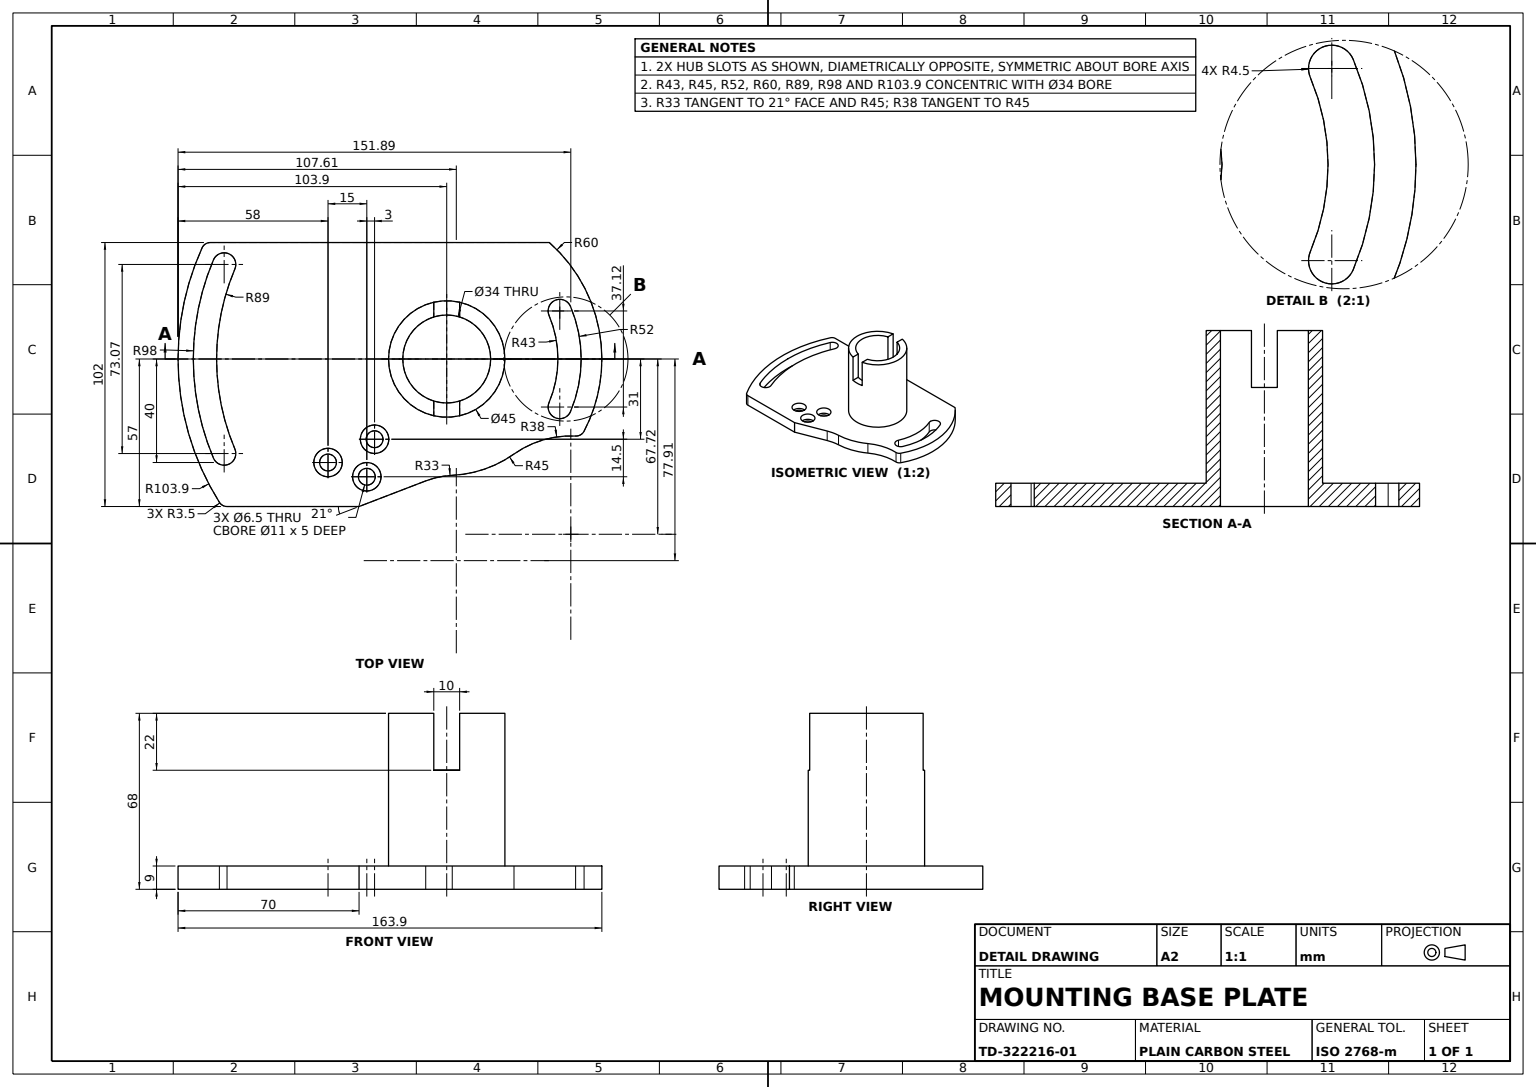
SolidWorks part; units mm, degrees
material "Plain Carbon Steel"
ref_plane "Front Plane" through (0, 0, 0) normal (0, 0, 1) x (1, 0, 0)
ref_plane "Top Plane" through (0, 0, 0) normal (0, 1, 0) x (1, 0, 0)
ref_plane "Right Plane" through (0, 0, 0) normal (1, 0, 0) x (0, 0, -1)
sketch "Cam Plate Profile" plane through (0, 0, 0) normal (0, 1, 0) x (1, 0, 0)
  line L0 (0, 0) -> (-45, 0) construction
  line L1 (-45, 39.6857) -> (-45, -91.4216)
  line L2 (0, 96.201) -> (0, -121.4761) construction
  line L3 (57, -84.9583) -> (57, -33.9)
  line L5 (0, 59.9996) -> (67.72, 59.9996) construction
  line L6 (57, -33.9) -> (47.1037, -8.1193)
  line L7 (57, -33.9) -> (57, 0) construction
  line L8 (65.0434, 47.9896) -> (85.4639, 47.9896) construction
  line L9 (67.72, 59.9996) -> (67.72, 47.9896) construction
  line L10 (0, -103.9) -> (-95.6382, -103.9) construction
  arc A0 (-42.9467, -94.6086) -> (55.365, -87.92) centre (0, 0) ccw
  arc A1 (-45, 39.6857) -> (27.8971, 53.1197) centre (0, 0) cw
  arc A2 (44.9492, 2.1386) -> (36.7157, 26.0185) centre (0, 0) ccw
  arc A3 (29.7656, 49.8497) -> (36.7157, 26.0185) centre (67.72, 47.9896) ccw
  arc A4 (29.7656, 49.8497) -> (27.8971, 53.1197) centre (26.2697, 50.021) ccw
  arc A5 (47.1037, -8.1193) -> (44.9492, 2.1386) centre (77.9119, 3.7068) cw
  arc A6 (57, -84.9583) -> (55.365, -87.92) centre (53.5, -84.9583) cw
  arc A7 (-45, -91.4216) -> (-42.9467, -94.6086) centre (-41.5, -91.4216) ccw
  dimension "D5" = 45
  dimension "D7" = 38
  dimension "D8" = 3.5
  dimension "D9" = 33
  dimension "D11" = 3.5
  dimension "D1" = 45
  dimension "D2" = 57
  dimension "D3" = 12.01
  dimension "D4" = 21
  dimension "D6" = 103.9
  dimension "D10" = 67.72
  dimension "D12" = 70
extrude "Cam Plate 9mm" add sketch "Cam Plate Profile" along normal blind 9
sketch "Arc Slots Profile" plane through (0, 9, 0) normal (0, 1, 0) x (1, 0, 0)
  line L0 (0, 0) -> (0, 77.1649) construction
  line L1 (0, 0) -> (-27.7764, 65.4371) construction
  line L2 (0, 0) -> (18.5597, 43.724) construction
  line L3 (0, 0) -> (0, -115.9598) construction
  line L4 (0, 0) -> (-36.5334, -86.0672) construction
  line L5 (0, 0) -> (36.5334, -86.0672) construction
  arc A0 (-18.5597, 43.724) -> (18.5597, 43.724) centre (0, 0) cw construction
  arc A1 (20.318, 47.8663) -> (-20.318, 47.8663) centre (0, 0) ccw
  arc A2 (16.8014, 39.5817) -> (-16.8014, 39.5817) centre (0, 0) ccw
  arc A3 (16.8014, 39.5817) -> (20.318, 47.8663) centre (18.5597, 43.724) ccw
  arc A4 (-20.318, 47.8663) -> (-16.8014, 39.5817) centre (-18.5597, 43.724) ccw
  arc A5 (36.5334, -86.0672) -> (-36.5334, -86.0672) centre (0, 0) cw construction
  arc A6 (-38.2917, -90.2095) -> (38.2917, -90.2095) centre (0, 0) ccw
  arc A7 (-34.7751, -81.9249) -> (34.7751, -81.9249) centre (0, 0) ccw
  arc A8 (-34.7751, -81.9249) -> (-38.2917, -90.2095) centre (-36.5334, -86.0672) ccw
  arc A9 (38.2917, -90.2095) -> (34.7751, -81.9249) centre (36.5334, -86.0672) ccw
  point P4 (0, 47.5)
  point P16 (0, -93.5)
  dimension "D1" = 47.5
  dimension "D2" = 9
  dimension "D5" = 9
  dimension "D6" = 93.5
  dimension "D3" = 23
  dimension "D4" = 23
extrude "Arc Slots" cut sketch "Arc Slots Profile" against normal up to next
sketch "Counterbore Hole Positions" plane through (0, 9, 0) normal (0, 1, 0) x (1, 0, 0)
  line L0 (0, 0) -> (0, -123.4243) construction
  line L1 (0, -27.9) -> (31, -27.9) construction
  line L2 (0, -45.9) -> (40, -45.9) construction
  line L3 (31, -27.9) -> (31, -30.9) construction
  line L4 (31, -30.9) -> (45.5, -30.9) construction
  line L5 (0, -103.9) -> (48.4187, -103.9) construction
  arc A0 (-42.9467, -94.6086) -> (55.365, -87.92) centre (0, 0) ccw construction
  dimension "D1" = 31
  dimension "D2" = 40
  dimension "D3" = 3
  dimension "D4" = 14.5
  dimension "D5" = 15
  dimension "D6" = 58
hole_wizard "Counterbored Holes Ø6.5" positions "3DSketch1" profile "Sketch4" legacy end condition up to next
sketch3d "3DSketch1"
  point P0 (31, 9, 27.9)
  point P3 (45.5, 9, 30.9)
  point P6 (40, 9, 45.9)
sketch "Sketch4" plane through (31, 9, 27.9) normal (1, 0, 0) x (0, 0, 1)
  line L0 (0, 0) -> (0, 9)
  line L1 (0, 9) -> (3.25, 9)
  line L2 (3.25, 9) -> (3.25, 5)
  line L3 (3.25, 5) -> (5.5, 5)
  line L4 (5.5, 5) -> (5.5, 0)
  line L5 (5.5, 0) -> (0, 0)
  line L6 (0, 110) -> (0, -10) construction
  dimension "Diameter" = 6.5
  dimension "Depth" = 9
  dimension "C-Bore Diameter" = 11
  dimension "C-Bore Depth" = 5
sketch "Hub Profile Ø45" plane through (0, 9, 0) normal (0, 1, 0) x (1, 0, 0)
  circle A0 centre (0, 0) radius 22.5
  dimension "D1" = 45
extrude "Hub Ø45" add sketch "Hub Profile Ø45" along normal blind 59
sketch "Hub Bore Profile Ø34" plane through (0, 68, 0) normal (0, 1, 0) x (1, 0, 0)
  circle A0 centre (0, 0) radius 17
  dimension "D1" = 34
extrude "Hub Bore Ø34" cut sketch "Hub Bore Profile Ø34" against normal through all
sketch "Hub Slots Profile" plane through (0, 68, 0) normal (0, 1, 0) x (1, 0, 0)
  line L1 (-22.5, -5) -> (22.5, -5)
  line L2 (-22.5, -5) -> (-22.5, 5)
  line L3 (-22.5, 5) -> (22.5, 5)
  line L4 (22.5, -5) -> (22.5, 5)
  line L5 (-22.5, -5) -> (22.5, 5) construction
  line L6 (-22.5, 5) -> (22.5, -5) construction
  circle A1 centre (0, 0) radius 22.5 construction
  point P0 (0, 0)
  dimension "D1" = 10
extrude "Hub Slots 10mm" cut sketch "Hub Slots Profile" against normal blind 22
